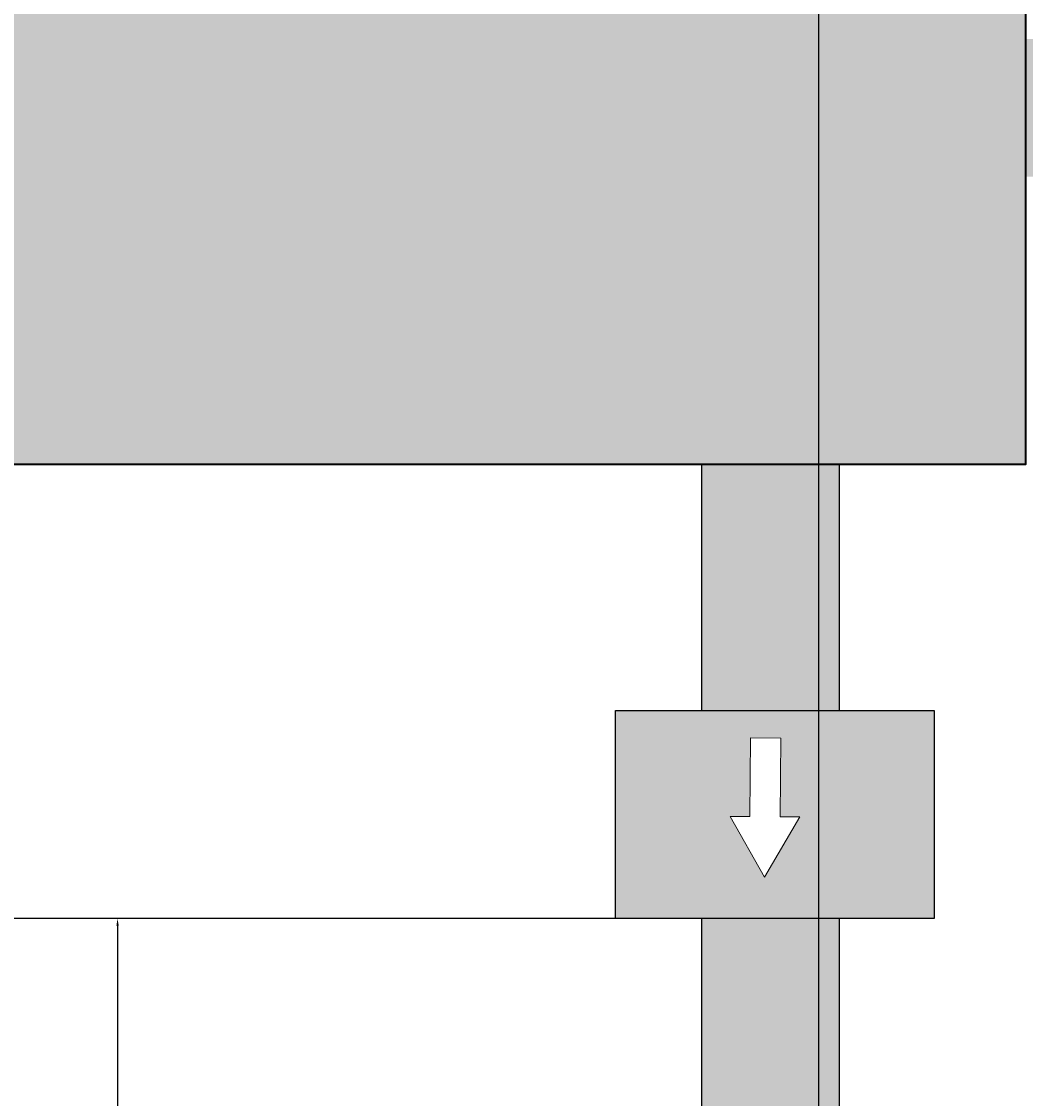
# Model space of a CAD drawing. Units: millimetres. Extents: x -11 to 280, y -4 to 208.
# Tile 51 of 55: x 211 to 237, y 129 to 156. Entities that reach past the tile are written whole.
import ezdxf

# ---------------------------------------------------------------- set-up
doc = ezdxf.new("R2010")
doc.units = ezdxf.units.MM
for name, color, linetype, lineweight in [('M-DIMS', 2, 'Continuous', 18), ('M-HYDR-EQPM', 7, 'Continuous', 35), ('M-HYDR-EQPM-PATT', 252, 'Continuous', 13), ('M-HYDR-PRES', 7, 'Continuous', 25), ('M-HYDR-SUCT', 7, 'Continuous', 25), ('M-HYDR-SYMB', 7, 'Continuous', 18), ('M-HYDR-VALV', 7, 'Continuous', 25)]:
    doc.layers.add(name, color=color, linetype=linetype, lineweight=lineweight)
doc.layers.add('M-HYDR-PRES-PATT', color=240, linetype='Continuous', lineweight=13, true_color=0xed1f24)
doc.layers.add('M-HYDR-SUCT-PATT', color=221, linetype='Continuous', lineweight=13, true_color=0xff7fdf)
doc.styles.get("Standard").update_dxf_attribs({"font": 'arial.ttf'})
doc.dimstyles.get("Standard").update_dxf_attribs({"dimtxt": 0.18, "dimasz": 0.18, "dimexe": 0.18, "dimexo": 0.0625, "dimgap": 0.09, "dimtad": 0, "dimtih": 1, "dimtoh": 1, "dimdec": 4, "dimzin": 0, "dimdsep": 46, "dimtxsty": 'Standard', "dimcen": 0.09, "dimadec": 0, "dimazin": 0, "dimtfac": 1, "dimtdec": 4, "dimtofl": 0, "dimtmove": 0, "dimatfit": 3, "dimfxl": 1, "dimtolj": 1, "dimtzin": 0, "dimarcsym": 0})

# ---------------------------------------------------------------- blocks, each defined once
blk = doc.blocks.new('HYDR-FLOW-ARROW')
for p, q in [((2, 1.272), (2, 1.772)), ((2, 1.772), (3.535, 0.886)), ((2, 1.272), (0, 1.272)), ((0, 1.272), (0, 0.5)), ((2, 0), (3.535, 0.886)), ((0, 0.5), (2, 0.5)), ((2, 0.5), (2, 0))]:
    blk.add_line(p, q)
blk = doc.blocks.new('*D5')
at = {"layer": 'Defpoints', "color": 0, "transparency": 16777216}
for p in [(24.759, 192.645), (-10.087, 11.435), (261.686, 11.435)]:
    blk.add_point(p, dxfattribs=at)
at = {"layer": 'M-DIMS', "color": 0, "lineweight": -2, "transparency": 16777216}
for p, q in [((24.696, 192.645), (-10.267, 192.645)), ((-10.087, 192.465), (-10.087, 102.222)), ((-10.087, 11.615), (-10.087, 101.858)), ((261.624, 11.435), (-10.267, 11.435))]:
    blk.add_line(p, q, dxfattribs=at)
at = {"layer": 'M-DIMS', "color": 0, "transparency": 16777216}
for points in [[(-10.117, 192.465), (-10.057, 192.465), (-10.087, 192.645)], [(-10.117, 11.615), (-10.057, 11.615), (-10.087, 11.435)]]:
    blk.add_solid(points, dxfattribs=at)
at = {"layer": 'M-DIMS', "color": 0, "transparency": 16777216, "insert": (-10.087, 102.04), "char_height": 0.18, "attachment_point": 5}
blk.add_mtext('\\A1;181.2', dxfattribs=at)
blk = doc.blocks.new('*D14')
at = {"layer": 'Defpoints', "color": 0, "transparency": 16777216}
for p in [(-10.087, 144.661), (205.531, 144.661), (226.511, 133.123)]:
    blk.add_point(p, dxfattribs=at)
at = {"layer": 'M-DIMS', "color": 0, "lineweight": -2, "transparency": 16777216}
for p, q in [((205.469, 144.661), (-10.267, 144.661)), ((-10.087, 144.481), (-10.087, 139.074)), ((-10.087, 133.303), (-10.087, 138.71)), ((226.448, 133.123), (-10.267, 133.123))]:
    blk.add_line(p, q, dxfattribs=at)
at = {"layer": 'M-DIMS', "color": 0, "transparency": 16777216}
for points in [[(-10.117, 144.481), (-10.057, 144.481), (-10.087, 144.661)], [(-10.117, 133.303), (-10.057, 133.303), (-10.087, 133.123)]]:
    blk.add_solid(points, dxfattribs=at)
at = {"layer": 'M-DIMS', "color": 0, "transparency": 16777216, "insert": (-10.087, 138.892), "char_height": 0.18, "attachment_point": 5}
blk.add_mtext('\\A1;11.538', dxfattribs=at)
blk = doc.blocks.new('*D15')
at = {"layer": 'Defpoints', "color": 0, "transparency": 16777216}
for p in [(213.85, 133.123), (228.7, 133.123), (228.7, 108.814)]:
    blk.add_point(p, dxfattribs=at)
at = {"layer": 'M-DIMS', "color": 0, "lineweight": -2, "transparency": 16777216}
for p, q in [((228.638, 133.123), (213.67, 133.123)), ((213.85, 132.943), (213.85, 121.15)), ((213.85, 108.994), (213.85, 120.786)), ((228.638, 108.814), (213.67, 108.814))]:
    blk.add_line(p, q, dxfattribs=at)
at = {"layer": 'M-DIMS', "color": 0, "transparency": 16777216}
for points in [[(213.82, 132.943), (213.88, 132.943), (213.85, 133.123)], [(213.82, 108.994), (213.88, 108.994), (213.85, 108.814)]]:
    blk.add_solid(points, dxfattribs=at)
at = {"layer": 'M-DIMS', "color": 0, "transparency": 16777216, "insert": (213.85, 120.968), "char_height": 0.18, "attachment_point": 5}
blk.add_mtext('\\A1;24.31', dxfattribs=at)
blk = doc.blocks.new('*D20')
at = {"layer": 'Defpoints', "color": 0, "transparency": 16777216}
for p in [(231.68, 207.495), (151.022, 43.599), (231.68, 43.599)]:
    blk.add_point(p, dxfattribs=at)
at = {"layer": 'M-DIMS', "color": 0, "lineweight": -2, "transparency": 16777216}
for p, q in [((151.022, 43.662), (151.022, 207.675)), ((151.202, 207.495), (190.957, 207.495)), ((231.5, 207.495), (191.745, 207.495)), ((231.68, 43.662), (231.68, 207.675))]:
    blk.add_line(p, q, dxfattribs=at)
at = {"layer": 'M-DIMS', "color": 0, "transparency": 16777216}
for points in [[(151.202, 207.525), (151.202, 207.465), (151.022, 207.495)], [(231.5, 207.525), (231.5, 207.465), (231.68, 207.495)]]:
    blk.add_solid(points, dxfattribs=at)
at = {"layer": 'M-DIMS', "color": 0, "transparency": 16777216, "insert": (191.351, 207.495), "char_height": 0.18, "attachment_point": 5}
blk.add_mtext('\\A1;80.66', dxfattribs=at)
blk = doc.blocks.new('*D22')
at = {"layer": 'Defpoints', "color": 0, "transparency": 16777216}
for p in [(259.871, 207.495), (231.68, 34.723), (259.871, 34.723)]:
    blk.add_point(p, dxfattribs=at)
at = {"layer": 'M-DIMS', "color": 0, "lineweight": -2, "transparency": 16777216}
for p, q in [((231.68, 34.785), (231.68, 207.675)), ((231.86, 207.495), (245.38, 207.495)), ((259.691, 207.495), (246.171, 207.495)), ((259.871, 34.785), (259.871, 207.675))]:
    blk.add_line(p, q, dxfattribs=at)
at = {"layer": 'M-DIMS', "color": 0, "transparency": 16777216}
for points in [[(231.86, 207.525), (231.86, 207.465), (231.68, 207.495)], [(259.691, 207.525), (259.691, 207.465), (259.871, 207.495)]]:
    blk.add_solid(points, dxfattribs=at)
at = {"layer": 'M-DIMS', "color": 0, "transparency": 16777216, "insert": (245.776, 207.495), "char_height": 0.18, "attachment_point": 5}
blk.add_mtext('\\A1;28.19', dxfattribs=at)

msp = doc.modelspace()

# ---------------------------------------------------------------- hatches: boundary and pattern name
at = {"layer": 'M-HYDR-EQPM-PATT'}
h = msp.add_hatch(color=256, dxfattribs=at)
h.set_gradient(color1=(248, 153, 30), color2=(248, 153, 30), tint=1)
h.paths.add_polyline_path([(236.9353, 165.103), (205.5315, 165.103), (205.5315, 144.6609), (236.9353, 144.6609)])
h.paths.add_polyline_path([(244.8074, 166.103), (205.5315, 166.103), (205.5315, 165.103), (236.9353, 165.103), (245.4299, 165.103)])
h.paths.add_polyline_path([(248.3313, 165.603, -0.4142136), (248.8313, 166.103), (245.9853, 166.103), (246.6078, 165.103), (248.8313, 165.103, -0.4142136)])
h.paths.add_polyline_path([(249.3313, 165.603, 1), (248.3313, 165.603, 0.4142136), (248.8313, 165.103, 0.4142136)])
at = {"layer": 'M-HYDR-PRES-PATT'}
h = msp.add_hatch(color=256, dxfattribs=at)
h.set_gradient(color1=(237, 31, 36), color2=(237, 31, 36), tint=1)
h.paths.add_polyline_path([(232.2, 133.1228), (228.7, 133.1228), (228.7, 108.8141), (102.7646, 108.8141), (102.7646, 105.3141), (232.2, 105.3141)])
h.paths.add_polyline_path([(128.8433, 105.3141), (125.3433, 105.3141), (125.3433, 91.7099, 1), (128.8433, 91.7099)])
h.paths.add_polyline_path([(229.1617, 78.7098), (196.7745, 78.7098, -0.4142136), (191.7745, 83.7098), (191.7745, 105.3141), (188.2745, 105.3141), (188.2745, 80.2098, 0.4142136), (193.2745, 75.2098), (225.6617, 75.2098), (225.6617, 43.5991), (229.1617, 43.5991)])
h.paths.add_polyline_path([(102.7646, 110.3704), (95.5776, 110.3704), (95.5776, 103.9022), (102.7646, 103.9022)])
h.paths.add_polyline_path([(100.7059, 107.2502), (99.1711, 106.3641), (99.1711, 106.8641), (97.1711, 106.8641), (97.1711, 107.6363), (99.1711, 107.6363), (99.1711, 108.1363)], flags=16)
h.paths.add_polyline_path([(234.6119, 138.4081), (226.5106, 138.4081), (226.5106, 133.1228), (234.6119, 133.1228)])
h.paths.add_polyline_path([(231.1963, 135.7055), (230.2965, 134.1786), (229.4241, 135.7213), (229.9241, 135.7168), (229.9418, 137.7167), (230.7141, 137.7099), (230.6963, 135.71)], flags=16)
at = {"layer": 'M-HYDR-SUCT-PATT'}
h = msp.add_hatch(color=256, dxfattribs=at)
h.set_gradient(color1=(255, 127, 223), color2=(255, 127, 223), tint=1, name='INVCYLINDER')
h.paths.add_polyline_path([(91.3629, 155.4768), (91.3629, 132.4768), (58.3629, 132.4768), (58.3629, 153.9768), (54.8629, 153.9768), (54.8629, 128.9768), (94.8629, 128.9768), (94.8629, 151.9768), (205.5315, 151.9768), (205.5315, 155.4768)])
h.paths.add_polyline_path([(91.3, 114.9452, 1), (78.8273, 114.9452), (78.8273, 108.8141), (42.6453, 108.8141), (42.6453, 153.9768), (39.1453, 153.9768), (39.1453, 105.3141), (78.8273, 105.3141), (78.8273, 98.1491, 1), (91.3, 98.1491), (91.3, 105.3141), (95.5776, 105.3141), (95.5776, 108.8141), (91.3, 108.8141)])
h.paths.add_polyline_path([(228.7, 138.4081), (232.2, 138.4081), (232.2, 144.6609), (228.7, 144.6609)])
h.paths.add_polyline_path([(253.1005, 151.9768, 1), (253.1005, 155.4768), (252.6001, 155.4768), (253.5249, 153.991, -0.1401047), (253.6005, 153.7268, -0.7542249), (252.676, 153.4626), (251.4221, 155.4768), (236.9353, 155.4768), (236.9353, 151.9768)])
h.paths.add_polyline_path([(30.8182, 40.7626), (30.8182, 36.7626), (60.8182, 36.7626), (60.8182, 40.7626)])

# ---------------------------------------------------------------- linework, layer by layer
at = {"layer": 'M-HYDR-EQPM'}
msp.add_lwpolyline([(205.5315, 165.103), (236.9353, 165.103), (236.9353, 144.6609), (205.5315, 144.6609)], close=True, dxfattribs=at)
at = {"layer": 'M-HYDR-PRES'}
for points in [[(232.2, 133.1228), (232.2, 105.3141), (102.7646, 105.3141)], [(228.7, 133.1228), (228.7, 108.8141), (102.7646, 108.8141)]]:
    msp.add_lwpolyline(points, dxfattribs=at)
at = {"layer": 'M-HYDR-SUCT'}
for points in [[(228.7, 144.6609), (228.7, 138.4081)], [(232.2, 144.6609), (232.2, 138.4081)]]:
    msp.add_lwpolyline(points, dxfattribs=at)
at = {"layer": 'M-HYDR-VALV'}
msp.add_lwpolyline([(226.5106, 138.4081), (234.6119, 138.4081), (234.6119, 133.1228), (226.5106, 133.1228)], close=True, dxfattribs=at)

# ---------------------------------------------------------------- block references
at = {"layer": 'M-HYDR-SYMB', "rotation": 269.4903545867307}
msp.add_blockref('HYDR-FLOW-ARROW', (229.4418, 137.7213), dxfattribs=at)

# ---------------------------------------------------------------- dimensions: what is measured, and where the dimension line sits
at = {"layer": 'M-DIMS'}
for base, p1, p2, picture, middle in [((231.6803, 207.495), (151.0217, 43.5991), (231.6803, 43.5991), '*D20', (191.351, 207.495)), ((259.871, 207.495), (231.6803, 34.7226), (259.871, 34.7226), '*D22', (245.7757, 207.495))]:
    dim = msp.add_linear_dim(base=base, p1=p1, p2=p2, dimstyle='Standard', override={"dimdec": 2, "dimlfac": 1, "dimrnd": 0, "dimzin": 0, "dimdsep": 46, "dimlunit": 2}, dxfattribs=at)
    dim.commit()
    dim.dimension.update_dxf_attribs({"geometry": picture, "text_midpoint": middle})
for base, p1, p2, override, picture, middle in [((-10.0865, 11.4346), (24.7588, 192.645), (261.6863, 11.4346), {"dimdec": 1, "dimlfac": 1, "dimrnd": 0, "dimzin": 0, "dimdsep": 46, "dimlunit": 2}, '*D5', (-10.0865, 102.0398)), ((-10.0865, 144.6609), (226.5106, 133.1228), (205.5315, 144.6609), {"dimdec": 3, "dimlfac": 1, "dimrnd": 0, "dimzin": 0, "dimdsep": 46, "dimlunit": 2}, '*D14', (-10.0865, 138.8918)), ((213.85, 133.1228), (228.7, 108.8141), (228.7, 133.1228), {"dimdec": 2, "dimlfac": 1, "dimrnd": 0, "dimzin": 0, "dimdsep": 46, "dimlunit": 2}, '*D15', (213.85, 120.9684))]:
    dim = msp.add_linear_dim(base=base, p1=p1, p2=p2, angle=90, dimstyle='Standard', override=override, dxfattribs=at)
    dim.commit()
    dim.dimension.update_dxf_attribs({"geometry": picture, "text_midpoint": middle})

doc.saveas('drawing.dxf')
